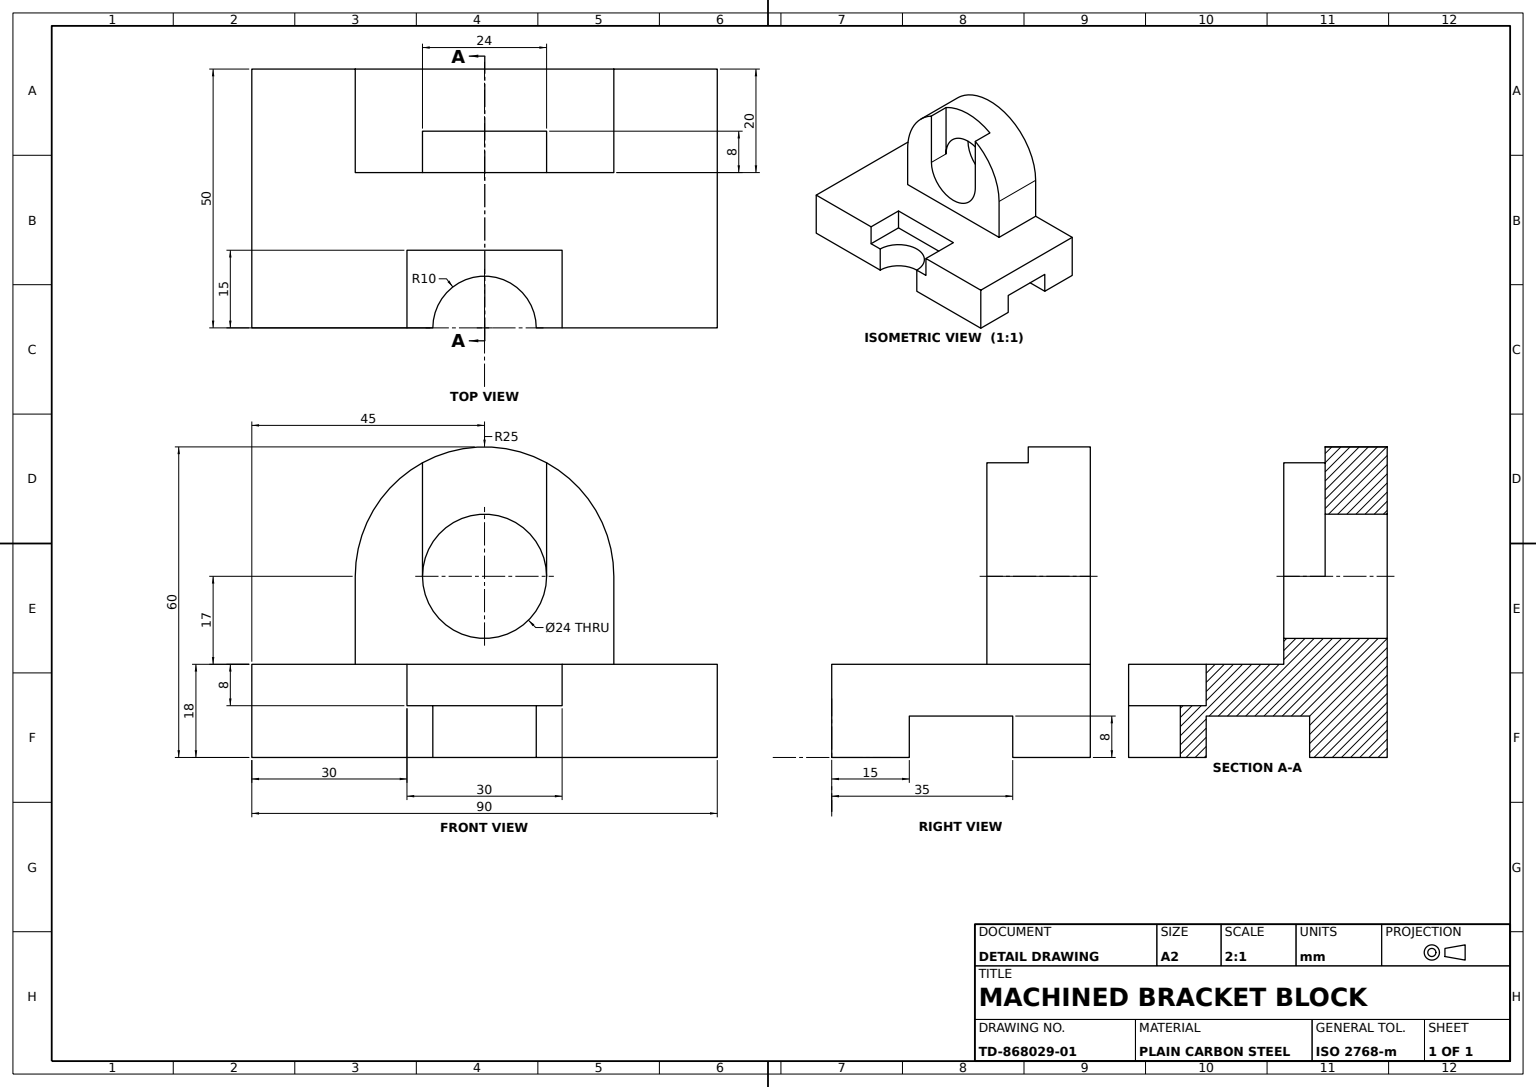
SolidWorks part; units mm, degrees
material "Plain Carbon Steel"
ref_plane "Front Plane" through (0, 0, 0) normal (0, 0, 1) x (1, 0, 0)
ref_plane "Top Plane" through (0, 0, 0) normal (0, 1, 0) x (1, 0, 0)
ref_plane "Right Plane" through (0, 0, 0) normal (1, 0, 0) x (0, 0, -1)
sketch "Base Plate Sketch" plane through (0, 0, 0) normal (0, 0, 1) x (1, 0, 0)
  line L0 (0, 0) -> (90, 0)
  line L1 (90, 0) -> (90, 18)
  line L2 (90, 18) -> (0, 18)
  line L3 (0, 18) -> (0, 0)
  dimension "D1" = 90
  dimension "D2" = 18
extrude "Base Plate 90x18x50" add sketch "Base Plate Sketch" along normal blind 50
ref_plane "Lug Face Plane" through (0, 0, 0) normal (0, 0, 1) x (1, 0, 0)
sketch "Pivot Lug Sketch" plane through (0, 0, 0) normal (0, 0, 1) x (1, 0, 0)
  line L0 (90, 18) -> (0, 18) construction
  line L1 (20, 35) -> (20, 18)
  line L2 (70, 35) -> (70, 18)
  line L3 (20, 18) -> (70, 18)
  circle A0 centre (45, 35) radius 12
  arc A1 (70, 35) -> (20, 35) centre (45, 35) ccw
  dimension "D1" = 17
  dimension "D4" = 24
  dimension "D2" = 45
  dimension "D3" = 50
extrude "Pivot Lug" add sketch "Pivot Lug Sketch" along normal blind 20
sketch "Bottom Groove Sketch" plane through (90, 0, 0) normal (1, 0, 0) x (0, 0, -1)
  line L0 (0, 0) -> (0, 18) construction
  line L1 (-35, 0) -> (-35, 8)
  line L2 (-35, 8) -> (-15, 8)
  line L3 (-15, 8) -> (-15, 0)
  line L4 (-50, 0) -> (0, 0) construction
  line L5 (-15, 0) -> (-35, 0)
  line L6 (-50, 18) -> (0, 18) construction
  dimension "D1" = 15
  dimension "D2" = 35
  dimension "D3" = 10
extrude "Bottom Groove" cut sketch "Bottom Groove Sketch" against normal through all
sketch "Lug Slot Sketch" plane through (0, 0, 20) normal (0, 0, 1) x (1, 0, 0)
  line L0 (33, 35) -> (33, 56.9317)
  line L1 (57, 35) -> (57, 56.9317)
  circle A0 centre (45, 35) radius 12 construction
  arc A1 (70, 35) -> (20, 35) centre (45, 35) ccw construction
  arc A2 (33, 56.9317) -> (57, 56.9317) centre (45, 35) cw
  arc A3 (33, 35) -> (57, 35) centre (45, 35) cw
extrude "Lug Slot" cut sketch "Lug Slot Sketch" against normal blind 8
sketch "Top Pocket Sketch" plane through (0, 18, 0) normal (0, 1, 0) x (1, 0, 0)
  line L0 (70, -20) -> (70, 0) construction
  line L1 (30, -35) -> (60, -35)
  line L2 (30, -35) -> (30, -50)
  line L3 (30, -50) -> (60, -50)
  line L4 (60, -35) -> (60, -50)
  line L5 (30, -35) -> (60, -50) construction
  line L6 (30, -50) -> (60, -35) construction
  line L7 (90, -50) -> (0, -50) construction
  point P0 (45, -50)
  dimension "D1" = 15
  dimension "D2" = 30
  dimension "D3" = 10
extrude "Top Pocket" cut sketch "Top Pocket Sketch" against normal blind 8
sketch "Pocket Hole Ø20 Sketch" plane through (0, 10, 0) normal (0, 1, 0) x (1, 0, 0)
  line L0 (30, -50) -> (60, -50) construction
  circle A0 centre (45, -50) radius 10
  dimension "D1" = 20
extrude "Pocket Hole Ø20" cut sketch "Pocket Hole Ø20 Sketch" against normal through all
